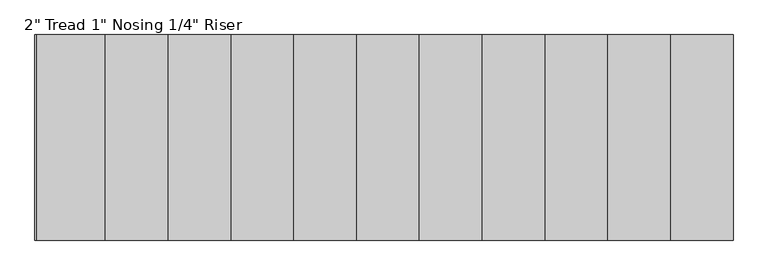
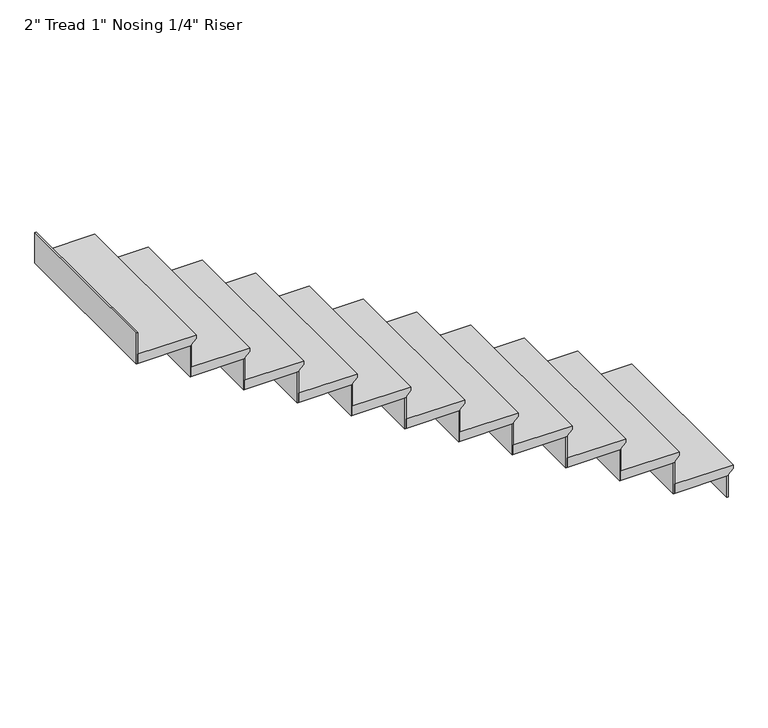
"""IFC4 building model written with IfcOpenShell, lengths in millimetres: stair flight geometry."""

from ifc_helpers import new_model, si_unit, origin, place, context, project, spatial, faceted_brep, source, transform, mapped, element, save


def stair_flight_cb879090(model_context):
    return source(origin(), model_context, "Body", "Brep", [
        faceted_brep([(-1385.5005972, 2819.495038, 150.2833333), (-1385.5005972, 2819.495038, 169.3333333), (-1385.5005972, 1905.095038, 169.3333333), (-1385.5005972, 1905.095038, 150.2833333), (-1410.9005972, 2819.495038, 124.8833333), (-1410.9005972, 1905.095038, 124.8833333), (-1690.3005972, 2819.495038, 169.3333333), (-1690.3005972, 1905.095038, 169.3333333), (-1410.9005972, 1905.095038, 118.5333333), (-1690.3005972, 1905.095038, 118.5333333), (-1690.3005972, 2819.495038, 118.5333333), (-1410.9005972, 2819.495038, 118.5333333)], [[[0, 1, 2, 3]], [[4, 0, 3, 5]], [[2, 1, 6, 7]], [[8, 9, 10, 11]], [[2, 7, 9, 8, 5, 3]], [[8, 11, 4, 5]], [[6, 1, 0, 4, 11, 10]], [[7, 6, 10, 9]]]),
        faceted_brep([(-1410.9005972, 2819.495038, 118.5333333), (-1410.9005972, 2819.495038, 0.0), (-1417.2505972, 2819.495038, 0.0), (-1417.2505972, 2819.495038, 118.5333333), (-1410.9005972, 1905.095038, 118.5333333), (-1417.2505972, 1905.095038, 118.5333333), (-1417.2505972, 1905.095038, 0.0), (-1410.9005972, 1905.095038, 0.0)], [[[0, 1, 2, 3]], [[4, 5, 6, 7]], [[1, 0, 4, 7]], [[2, 1, 7, 6]], [[3, 2, 6, 5]], [[0, 3, 5, 4]]]),
        faceted_brep([(-1690.3005972, 2819.495038, 287.8666667), (-1690.3005972, 2819.495038, 118.5333333), (-1696.6505972, 2819.495038, 118.5333333), (-1696.6505972, 2819.495038, 287.8666667), (-1690.3005972, 1905.095038, 287.8666667), (-1696.6505972, 1905.095038, 287.8666667), (-1696.6505972, 1905.095038, 118.5333333), (-1690.3005972, 1905.095038, 118.5333333)], [[[0, 1, 2, 3]], [[4, 5, 6, 7]], [[1, 0, 4, 7]], [[2, 1, 7, 6]], [[3, 2, 6, 5]], [[0, 3, 5, 4]]]),
        faceted_brep([(-1664.9005972, 1905.095038, 338.6666667), (-1664.9005972, 2819.495038, 338.6666667), (-1969.7005972, 2819.495038, 338.6666667), (-1969.7005972, 1905.095038, 338.6666667), (-1690.3005972, 1905.095038, 287.8666667), (-1969.7005972, 1905.095038, 287.8666667), (-1969.7005972, 2819.495038, 287.8666667), (-1690.3005972, 2819.495038, 287.8666667), (-1690.3005972, 1905.095038, 294.2166667), (-1664.9005972, 1905.095038, 319.6166667), (-1690.3005972, 2819.495038, 294.2166667), (-1664.9005972, 2819.495038, 319.6166667)], [[[0, 1, 2, 3]], [[4, 5, 6, 7]], [[0, 3, 5, 4, 8, 9]], [[4, 7, 10, 8]], [[2, 1, 11, 10, 7, 6]], [[3, 2, 6, 5]], [[11, 1, 0, 9]], [[10, 11, 9, 8]]]),
        faceted_brep([(-1969.7005972, 2819.495038, 457.2), (-1969.7005972, 2819.495038, 287.8666667), (-1976.0505972, 2819.495038, 287.8666667), (-1976.0505972, 2819.495038, 457.2), (-1969.7005972, 1905.095038, 457.2), (-1976.0505972, 1905.095038, 457.2), (-1976.0505972, 1905.095038, 287.8666667), (-1969.7005972, 1905.095038, 287.8666667)], [[[0, 1, 2, 3]], [[4, 5, 6, 7]], [[1, 0, 4, 7]], [[2, 1, 7, 6]], [[3, 2, 6, 5]], [[0, 3, 5, 4]]]),
        faceted_brep([(-1944.3005972, 1905.095038, 508.0), (-1944.3005972, 2819.495038, 508.0), (-2249.1005972, 2819.495038, 508.0), (-2249.1005972, 1905.095038, 508.0), (-1969.7005972, 1905.095038, 457.2), (-2249.1005972, 1905.095038, 457.2), (-2249.1005972, 2819.495038, 457.2), (-1969.7005972, 2819.495038, 457.2), (-1969.7005972, 1905.095038, 463.55), (-1944.3005972, 1905.095038, 488.95), (-1969.7005972, 2819.495038, 463.55), (-1944.3005972, 2819.495038, 488.95)], [[[0, 1, 2, 3]], [[4, 5, 6, 7]], [[0, 3, 5, 4, 8, 9]], [[4, 7, 10, 8]], [[2, 1, 11, 10, 7, 6]], [[3, 2, 6, 5]], [[11, 1, 0, 9]], [[10, 11, 9, 8]]]),
        faceted_brep([(-2249.1005972, 2819.495038, 626.5333333), (-2249.1005972, 2819.495038, 457.2), (-2255.4505972, 2819.495038, 457.2), (-2255.4505972, 2819.495038, 626.5333333), (-2249.1005972, 1905.095038, 626.5333333), (-2255.4505972, 1905.095038, 626.5333333), (-2255.4505972, 1905.095038, 457.2), (-2249.1005972, 1905.095038, 457.2)], [[[0, 1, 2, 3]], [[4, 5, 6, 7]], [[1, 0, 4, 7]], [[2, 1, 7, 6]], [[3, 2, 6, 5]], [[0, 3, 5, 4]]]),
        faceted_brep([(-2223.7005972, 1905.095038, 677.3333333), (-2223.7005972, 2819.495038, 677.3333333), (-2528.5005972, 2819.495038, 677.3333333), (-2528.5005972, 1905.095038, 677.3333333), (-2249.1005972, 1905.095038, 626.5333333), (-2528.5005972, 1905.095038, 626.5333333), (-2528.5005972, 2819.495038, 626.5333333), (-2249.1005972, 2819.495038, 626.5333333), (-2249.1005972, 1905.095038, 632.8833333), (-2223.7005972, 1905.095038, 658.2833333), (-2249.1005972, 2819.495038, 632.8833333), (-2223.7005972, 2819.495038, 658.2833333)], [[[0, 1, 2, 3]], [[4, 5, 6, 7]], [[0, 3, 5, 4, 8, 9]], [[4, 7, 10, 8]], [[2, 1, 11, 10, 7, 6]], [[3, 2, 6, 5]], [[11, 1, 0, 9]], [[10, 11, 9, 8]]]),
        faceted_brep([(-2528.5005972, 2819.495038, 795.8666667), (-2528.5005972, 2819.495038, 626.5333333), (-2534.8505972, 2819.495038, 626.5333333), (-2534.8505972, 2819.495038, 795.8666667), (-2528.5005972, 1905.095038, 795.8666667), (-2534.8505972, 1905.095038, 795.8666667), (-2534.8505972, 1905.095038, 626.5333333), (-2528.5005972, 1905.095038, 626.5333333)], [[[0, 1, 2, 3]], [[4, 5, 6, 7]], [[1, 0, 4, 7]], [[2, 1, 7, 6]], [[3, 2, 6, 5]], [[0, 3, 5, 4]]]),
        faceted_brep([(-2503.1005972, 1905.095038, 846.6666667), (-2503.1005972, 2819.495038, 846.6666667), (-2807.9005972, 2819.495038, 846.6666667), (-2807.9005972, 1905.095038, 846.6666667), (-2528.5005972, 1905.095038, 795.8666667), (-2807.9005972, 1905.095038, 795.8666667), (-2807.9005972, 2819.495038, 795.8666667), (-2528.5005972, 2819.495038, 795.8666667), (-2528.5005972, 1905.095038, 802.2166667), (-2503.1005972, 1905.095038, 827.6166667), (-2528.5005972, 2819.495038, 802.2166667), (-2503.1005972, 2819.495038, 827.6166667)], [[[0, 1, 2, 3]], [[4, 5, 6, 7]], [[0, 3, 5, 4, 8, 9]], [[4, 7, 10, 8]], [[2, 1, 11, 10, 7, 6]], [[3, 2, 6, 5]], [[11, 1, 0, 9]], [[10, 11, 9, 8]]]),
        faceted_brep([(-2807.9005972, 2819.495038, 965.2), (-2807.9005972, 2819.495038, 795.8666667), (-2814.2505972, 2819.495038, 795.8666667), (-2814.2505972, 2819.495038, 965.2), (-2807.9005972, 1905.095038, 965.2), (-2814.2505972, 1905.095038, 965.2), (-2814.2505972, 1905.095038, 795.8666667), (-2807.9005972, 1905.095038, 795.8666667)], [[[0, 1, 2, 3]], [[4, 5, 6, 7]], [[1, 0, 4, 7]], [[2, 1, 7, 6]], [[3, 2, 6, 5]], [[0, 3, 5, 4]]]),
        faceted_brep([(-2782.5005972, 1905.095038, 1016.0), (-2782.5005972, 2819.495038, 1016.0), (-3087.3005972, 2819.495038, 1016.0), (-3087.3005972, 1905.095038, 1016.0), (-2807.9005972, 1905.095038, 965.2), (-3087.3005972, 1905.095038, 965.2), (-3087.3005972, 2819.495038, 965.2), (-2807.9005972, 2819.495038, 965.2), (-2807.9005972, 1905.095038, 971.55), (-2782.5005972, 1905.095038, 996.95), (-2807.9005972, 2819.495038, 971.55), (-2782.5005972, 2819.495038, 996.95)], [[[0, 1, 2, 3]], [[4, 5, 6, 7]], [[0, 3, 5, 4, 8, 9]], [[4, 7, 10, 8]], [[2, 1, 11, 10, 7, 6]], [[3, 2, 6, 5]], [[11, 1, 0, 9]], [[10, 11, 9, 8]]]),
        faceted_brep([(-3087.3005972, 2819.495038, 1134.5333333), (-3087.3005972, 2819.495038, 965.2), (-3093.6505972, 2819.495038, 965.2), (-3093.6505972, 2819.495038, 1134.5333333), (-3087.3005972, 1905.095038, 1134.5333333), (-3093.6505972, 1905.095038, 1134.5333333), (-3093.6505972, 1905.095038, 965.2), (-3087.3005972, 1905.095038, 965.2)], [[[0, 1, 2, 3]], [[4, 5, 6, 7]], [[1, 0, 4, 7]], [[2, 1, 7, 6]], [[3, 2, 6, 5]], [[0, 3, 5, 4]]]),
        faceted_brep([(-3061.9005972, 1905.095038, 1185.3333333), (-3061.9005972, 2819.495038, 1185.3333333), (-3366.7005972, 2819.495038, 1185.3333333), (-3366.7005972, 1905.095038, 1185.3333333), (-3087.3005972, 1905.095038, 1134.5333333), (-3366.7005972, 1905.095038, 1134.5333333), (-3366.7005972, 2819.495038, 1134.5333333), (-3087.3005972, 2819.495038, 1134.5333333), (-3087.3005972, 1905.095038, 1140.8833333), (-3061.9005972, 1905.095038, 1166.2833333), (-3087.3005972, 2819.495038, 1140.8833333), (-3061.9005972, 2819.495038, 1166.2833333)], [[[0, 1, 2, 3]], [[4, 5, 6, 7]], [[0, 3, 5, 4, 8, 9]], [[4, 7, 10, 8]], [[2, 1, 11, 10, 7, 6]], [[3, 2, 6, 5]], [[11, 1, 0, 9]], [[10, 11, 9, 8]]]),
        faceted_brep([(-3366.7005972, 2819.495038, 1303.8666667), (-3366.7005972, 2819.495038, 1134.5333333), (-3373.0505972, 2819.495038, 1134.5333333), (-3373.0505972, 2819.495038, 1303.8666667), (-3366.7005972, 1905.095038, 1303.8666667), (-3373.0505972, 1905.095038, 1303.8666667), (-3373.0505972, 1905.095038, 1134.5333333), (-3366.7005972, 1905.095038, 1134.5333333)], [[[0, 1, 2, 3]], [[4, 5, 6, 7]], [[1, 0, 4, 7]], [[2, 1, 7, 6]], [[3, 2, 6, 5]], [[0, 3, 5, 4]]]),
        faceted_brep([(-3341.3005972, 1905.095038, 1354.6666667), (-3341.3005972, 2819.495038, 1354.6666667), (-3646.1005972, 2819.495038, 1354.6666667), (-3646.1005972, 1905.095038, 1354.6666667), (-3366.7005972, 1905.095038, 1303.8666667), (-3646.1005972, 1905.095038, 1303.8666667), (-3646.1005972, 2819.495038, 1303.8666667), (-3366.7005972, 2819.495038, 1303.8666667), (-3366.7005972, 1905.095038, 1310.2166667), (-3341.3005972, 1905.095038, 1335.6166667), (-3366.7005972, 2819.495038, 1310.2166667), (-3341.3005972, 2819.495038, 1335.6166667)], [[[0, 1, 2, 3]], [[4, 5, 6, 7]], [[0, 3, 5, 4, 8, 9]], [[4, 7, 10, 8]], [[2, 1, 11, 10, 7, 6]], [[3, 2, 6, 5]], [[11, 1, 0, 9]], [[10, 11, 9, 8]]]),
        faceted_brep([(-3646.1005972, 2819.495038, 1473.2), (-3646.1005972, 2819.495038, 1303.8666667), (-3652.4505972, 2819.495038, 1303.8666667), (-3652.4505972, 2819.495038, 1473.2), (-3646.1005972, 1905.095038, 1473.2), (-3652.4505972, 1905.095038, 1473.2), (-3652.4505972, 1905.095038, 1303.8666667), (-3646.1005972, 1905.095038, 1303.8666667)], [[[0, 1, 2, 3]], [[4, 5, 6, 7]], [[1, 0, 4, 7]], [[2, 1, 7, 6]], [[3, 2, 6, 5]], [[0, 3, 5, 4]]]),
        faceted_brep([(-3620.7005972, 1905.095038, 1524.0), (-3620.7005972, 2819.495038, 1524.0), (-3925.5005972, 2819.495038, 1524.0), (-3925.5005972, 1905.095038, 1524.0), (-3646.1005972, 1905.095038, 1473.2), (-3925.5005972, 1905.095038, 1473.2), (-3925.5005972, 2819.495038, 1473.2), (-3646.1005972, 2819.495038, 1473.2), (-3646.1005972, 1905.095038, 1479.55), (-3620.7005972, 1905.095038, 1504.95), (-3646.1005972, 2819.495038, 1479.55), (-3620.7005972, 2819.495038, 1504.95)], [[[0, 1, 2, 3]], [[4, 5, 6, 7]], [[0, 3, 5, 4, 8, 9]], [[4, 7, 10, 8]], [[2, 1, 11, 10, 7, 6]], [[3, 2, 6, 5]], [[11, 1, 0, 9]], [[10, 11, 9, 8]]]),
        faceted_brep([(-3925.5005972, 2819.495038, 1642.5333333), (-3925.5005972, 2819.495038, 1473.2), (-3931.8505972, 2819.495038, 1473.2), (-3931.8505972, 2819.495038, 1642.5333333), (-3925.5005972, 1905.095038, 1642.5333333), (-3931.8505972, 1905.095038, 1642.5333333), (-3931.8505972, 1905.095038, 1473.2), (-3925.5005972, 1905.095038, 1473.2)], [[[0, 1, 2, 3]], [[4, 5, 6, 7]], [[1, 0, 4, 7]], [[2, 1, 7, 6]], [[3, 2, 6, 5]], [[0, 3, 5, 4]]]),
        faceted_brep([(-3900.1005972, 1905.095038, 1693.3333333), (-3900.1005972, 2819.495038, 1693.3333333), (-4204.9005972, 2819.495038, 1693.3333333), (-4204.9005972, 1905.095038, 1693.3333333), (-3925.5005972, 1905.095038, 1642.5333333), (-4204.9005972, 1905.095038, 1642.5333333), (-4204.9005972, 2819.495038, 1642.5333333), (-3925.5005972, 2819.495038, 1642.5333333), (-3925.5005972, 1905.095038, 1648.8833333), (-3900.1005972, 1905.095038, 1674.2833333), (-3925.5005972, 2819.495038, 1648.8833333), (-3900.1005972, 2819.495038, 1674.2833333)], [[[0, 1, 2, 3]], [[4, 5, 6, 7]], [[0, 3, 5, 4, 8, 9]], [[4, 7, 10, 8]], [[2, 1, 11, 10, 7, 6]], [[3, 2, 6, 5]], [[11, 1, 0, 9]], [[10, 11, 9, 8]]]),
        faceted_brep([(-4484.3005972, 2819.495038, 1981.2), (-4484.3005972, 2819.495038, 1811.8666667), (-4490.6505972, 2819.495038, 1811.8666667), (-4490.6505972, 2819.495038, 1981.2), (-4484.3005972, 1905.095038, 1981.2), (-4490.6505972, 1905.095038, 1981.2), (-4490.6505972, 1905.095038, 1811.8666667), (-4484.3005972, 1905.095038, 1811.8666667)], [[[0, 1, 2, 3]], [[4, 5, 6, 7]], [[1, 0, 4, 7]], [[2, 1, 7, 6]], [[3, 2, 6, 5]], [[0, 3, 5, 4]]]),
        faceted_brep([(-4204.9005972, 2819.495038, 1811.8666667), (-4204.9005972, 2819.495038, 1642.5333333), (-4211.2505972, 2819.495038, 1642.5333333), (-4211.2505972, 2819.495038, 1811.8666667), (-4204.9005972, 1905.095038, 1811.8666667), (-4211.2505972, 1905.095038, 1811.8666667), (-4211.2505972, 1905.095038, 1642.5333333), (-4204.9005972, 1905.095038, 1642.5333333)], [[[0, 1, 2, 3]], [[4, 5, 6, 7]], [[1, 0, 4, 7]], [[2, 1, 7, 6]], [[3, 2, 6, 5]], [[0, 3, 5, 4]]]),
        faceted_brep([(-4179.5005972, 1905.095038, 1862.6666667), (-4179.5005972, 2819.495038, 1862.6666667), (-4458.9005972, 2819.495038, 1862.6666667), (-4484.3005972, 2819.495038, 1862.6666667), (-4484.3005972, 1905.095038, 1862.6666667), (-4204.9005972, 1905.095038, 1811.8666667), (-4484.3005972, 1905.095038, 1811.8666667), (-4484.3005972, 2819.495038, 1811.8666667), (-4458.9005972, 2819.495038, 1811.8666667), (-4204.9005972, 2819.495038, 1811.8666667), (-4204.9005972, 1905.095038, 1818.2166667), (-4179.5005972, 1905.095038, 1843.6166667), (-4204.9005972, 2819.495038, 1818.2166667), (-4179.5005972, 2819.495038, 1843.6166667)], [[[0, 1, 2, 3, 4]], [[5, 6, 7, 8, 9]], [[0, 4, 6, 5, 10, 11]], [[5, 9, 12, 10]], [[2, 1, 13, 12, 9, 8]], [[3, 2, 8, 7]], [[4, 3, 7, 6]], [[13, 1, 0, 11]], [[12, 13, 11, 10]]]),
    ])


if __name__ == "__main__":
    model = new_model("IFC4")
    model_context = context("Model", 3, world=origin())
    ifc_project = project(units=[si_unit("LENGTHUNIT", "METRE", prefix="MILLI")], contexts=[model_context])
    site = spatial("IfcSite", under=ifc_project)
    building = spatial("IfcBuilding", under=site)
    placement = place(None, origin())
    stair_flight_shape = stair_flight_cb879090(model_context)
    element("IfcStairFlight", 1, ObjectType="2\" Tread 1\" Nosing 1/4\" Riser", at=placement, inside=building, context=model_context, shape_type="MappedRepresentation", body=[
        mapped(stair_flight_shape, transform((0.0, 0.0, 0.0), x_axis=(1.0, 0.0, 0.0), y_axis=(0.0, 1.0, 0.0), z_axis=(0.0, 0.0, 1.0))),
    ])
    save(model, "model.ifc")

# Revit data of these elements
# Element 1 (IfcStairFlight, "2\" Tread 1\" Nosing 1/4\" Riser")
#   Materials on its faces: "Gypsum Wall Board"
# Materials
#   "Gypsum Wall Board": class "Generic", colour RGB 127 127 127, transparency 0, Description = "Gypsum Wall Board", Cost = 0
